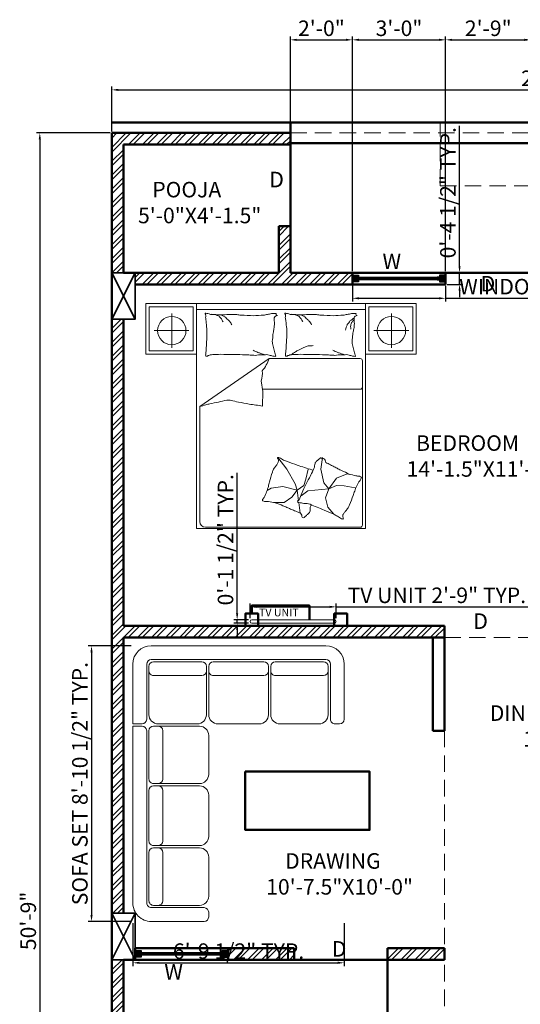
# Model space of a CAD drawing. Units: millimetres. Extents: x 67033 to 68301, y 155969 to 157209.
# Tile 4 of 17: x 67033 to 67226, y 156800 to 157181. Entities that reach past the tile are written whole.
import ezdxf

# ---------------------------------------------------------------- set-up
doc = ezdxf.new("R2010")
doc.units = ezdxf.units.MM
doc.linetypes.add('HIDDEN', pattern=[9.525, 6.35, -3.175])
for name, color, linetype, lineweight in [('A-ANNO-DIMS', 2, 'Continuous', 18), ('A-ANNO-TEXT', 7, 'Continuous', 18), ('A-AREA-IDEN', 3, 'Continuous', 18), ('A-COLS', 3, 'Continuous', 35), ('A-FLOR-OVHD', 1, 'HIDDEN', 18), ('A-FURN', 8, 'Continuous', 18), ('A-GLAZ', 4, 'Continuous', 25), ('A-WALL', 7, 'Continuous', 50), ('A-WALL-PATT', 8, 'Continuous', 13)]:
    doc.layers.add(name, color=color, linetype=linetype, lineweight=lineweight)
doc.styles.add('DIM_FONT', font='SIMPLEX.shx', dxfattribs={"width": 0.8})
doc.styles.get("Standard").update_dxf_attribs({"font": 'arial.ttf'})
doc.dimstyles.new('ISO-25', dxfattribs={"dimtxt": 6, "dimasz": 2.5, "dimexe": 1.25, "dimexo": 0.625, "dimtad": 1, "dimdec": 0, "dimlunit": 3, "dimtxsty": 'Standard', "dimcen": 2.5, "dimadec": 0, "dimazin": 0, "dimtfac": 1, "dimtdec": 0, "dimtmove": 0, "dimatfit": 3, "dimfxl": 1, "dimarcsym": 0})

# ---------------------------------------------------------------- blocks, each defined once
blk = doc.blocks.new('A$C79766A75')
for p, q in [((0.45, 1.9999), (0, 1.9999)), ((0, 1.9999), (0, 1.5499)), ((0.42, 1.9699), (0.03, 1.9699)), ((0.03, 1.9699), (0.03, 1.5799)), ((0.42, 1.5799), (0.42, 1.9699)), ((0.45, 1.5499), (0.45, 1.9999)), ((1.9506, 2), (0.4506, 2)), ((0.4506, 2), (0.4506, 0)), ((1.9506, 1.9476), (0.4506, 1.9476)), ((1.9506, 0), (1.9506, 2)), ((2.402, 1.9999), (1.952, 1.9999)), ((1.952, 1.9999), (1.952, 1.5499)), ((2.372, 1.9699), (1.982, 1.9699)), ((1.982, 1.9699), (1.982, 1.5799)), ((2.372, 1.5799), (2.372, 1.9699)), ((2.402, 1.5499), (2.402, 1.9999)), ((0.2304, 1.9125), (0.2304, 1.6061)), ((2.1824, 1.9125), (2.1824, 1.6061)), ((0.0743, 1.7595), (0.3834, 1.7595)), ((2.0263, 1.7595), (2.3354, 1.7595)), ((0.03, 1.5799), (0.42, 1.5799)), ((0.4234, 1.6034), (0.4228, 1.6034)), ((1.1461, 1.5617), (1.1254, 1.6443)), ((1.8553, 1.5617), (1.8346, 1.6443)), ((1.982, 1.5799), (2.372, 1.5799)), ((0, 1.5499), (0.45, 1.5499)), ((1.0972, 1.5115), (0.4791, 1.0841)), ((1.0972, 1.5115), (1.9048, 1.5115)), ((1.1536, 1.5317), (1.1461, 1.5617)), ((1.8628, 1.5317), (1.8553, 1.5617)), ((1.9248, 1.4915), (1.9248, 0.0322)), ((1.952, 1.5499), (2.402, 1.5499)), ((1.0383, 1.2184), (1.0246, 1.3138)), ((1.9048, 1.2389), (1.0354, 1.2389)), ((1.0365, 1.0883), (1.0383, 1.2184)), ((0.4791, 0.0622), (0.4791, 1.0841)), ((1.1731, 0.6316), (1.2523, 0.5276)), ((1.5696, 0.6317), (1.5559, 0.5286)), ((1.2523, 0.5276), (1.3274, 0.3973)), ((1.4223, 0.4407), (1.442, 0.5296)), ((1.5559, 0.5286), (1.5817, 0.4065)), ((1.4025, 0.3834), (1.4223, 0.4407)), ((1.6264, 0.355), (1.6952, 0.4478)), ((1.6952, 0.4478), (1.7898, 0.4856)), ((1.7898, 0.4856), (1.8139, 0.4822)), ((1.1139, 0.3597), (1.0779, 0.3397)), ((1.2167, 0.3736), (1.1139, 0.3597)), ((1.3452, 0.342), (1.2167, 0.3736)), ((1.3274, 0.3973), (1.3452, 0.342)), ((1.3452, 0.342), (1.4025, 0.3834)), ((1.4034, 0.3558), (1.3803, 0.2995)), ((1.6264, 0.355), (1.4406, 0.3361)), ((1.5817, 0.4065), (1.6264, 0.355)), ((1.5954, 0.2725), (1.6264, 0.355)), ((1.6264, 0.355), (1.6935, 0.3825)), ((1.6935, 0.3825), (1.7623, 0.379)), ((1.7623, 0.379), (1.8603, 0.3619)), ((1.8603, 0.3619), (1.8636, 0.3554)), ((1.2305, 0.2313), (1.2957, 0.2787)), ((1.2957, 0.2787), (1.3452, 0.342)), ((1.3452, 0.342), (1.3569, 0.2478)), ((1.3803, 0.2995), (1.3626, 0.256)), ((1.3907, 0.3), (1.3787, 0.2914)), ((1.4406, 0.3361), (1.3907, 0.3)), ((1.6161, 0.19), (1.5954, 0.2725)), ((1.1376, 0.2313), (1.2305, 0.2313)), ((1.3588, 0.2331), (1.3706, 0.1385)), ((1.6697, 0.1274), (1.6161, 0.19)), ((1.9048, 0.0122), (0.5291, 0.0122)), ((0.4506, 0), (1.9506, 0))]:
    blk.add_line(p, q)
for centre in [(0.2304, 1.7595), (2.1824, 1.7595)]:
    blk.add_circle(centre, 0.126)
for centre, radius, start, end in [((0.5232, 1.9139), 0.00342, 291.7883, 340.43603), ((0.525, 1.9085), 0.00232, 340.43603, 101.89306), ((0.5246, 1.9378), 0.0251, 274.30254, 291.7883), ((0.5311, 1.9093), 0.00428, 201.9904, 281.89306), ((0.4996, 1.8889), 0.0328, 338.57902, 8.13348), ((0.2896, 1.8253), 0.246, 8.13348, 12.10946), ((0.5465, 1.8994), 0.0156, 158.57902, 201.9904), ((0.7297, 1.8867), 0.1983, 187.6809, 192.10946), ((0.5486, 1.9393), 0.0289, 239.34875, 274.30254), ((1.4472, 1.8987), 0.9131, 183.36875, 187.6809), ((0.5458, 1.8568), 0.0539, 59.34875, 84.74081), ((0.546, 1.0829), 0.8208, 84.74081, 88.09211), ((0.6118, 2.0005), 0.0992, 254.06476, 274.21588), ((0.6775, 1.9817), 0.0992, 233.91364, 254.06476), ((0.6362, 0.406), 1.4943, 88.09211, 90.57574), ((0.7304, 1.9449), 0.0992, 216.17665, 233.91364), ((0.7737, 2.1075), 0.234, 242.76041, 249.13972), ((0.7661, 1.8961), 0.0992, 198.43965, 216.17665), ((0.7591, 1.0293), 0.8732, 90.57574, 94.80185), ((0.738, 1.949), 0.0768, 231.61143, 242.76041), ((0.974, 2.1633), 0.3916, 226.18849, 231.61143), ((0.9057, 1.9982), 0.2252, 219.03494, 226.18849), ((0.7631, 2.1919), 0.2897, 267.46141, 274.80185), ((0.8143, 2.0532), 0.1524, 259.81012, 267.46141), ((0.7515, 1.3747), 0.5293, 79.81012, 83.9133), ((0.8451, 0.8466), 1.049, 83.9133, 90), ((1.046, 1.2129), 0.6827, 90, 97.54685), ((1.1117, 1.6625), 0.2422, 97.54685, 105.74398), ((1.0352, 2.2041), 0.3048, 278.43719, 285.74398), ((1.1179, 2.0719), 0.1611, 270, 278.43719), ((1.171, 1.8579), 0.0342, 94.40021, 153.41948), ((1.6324, 1.8735), 0.4918, 180, 186.23236), ((1.1592, 2.0011), 0.0904, 258.72762, 270), ((1.1709, 1.9049), 0.0131, 153.41948, 258.72762), ((1.2325, 1.9139), 0.00342, 291.7883, 340.43603), ((1.2342, 1.9085), 0.00232, 340.43603, 101.89306), ((1.2338, 1.9378), 0.0251, 274.30254, 291.7883), ((1.2404, 1.9093), 0.00428, 201.9904, 281.89306), ((1.2088, 1.8889), 0.0328, 338.57902, 8.13348), ((0.9988, 1.8253), 0.246, 8.13348, 12.10946), ((1.2558, 1.8994), 0.0156, 158.57902, 201.9904), ((1.4389, 1.8867), 0.1983, 187.6809, 192.10946), ((1.2578, 1.9393), 0.0289, 239.34875, 274.30254), ((2.1565, 1.8987), 0.9131, 183.36875, 187.6809), ((1.2551, 1.8568), 0.0539, 59.34875, 84.74081), ((1.2552, 1.0829), 0.8208, 84.74081, 88.09211), ((1.3211, 2.0005), 0.0992, 254.06476, 274.21588), ((1.3868, 1.9817), 0.0992, 233.91364, 254.06476), ((1.3455, 0.406), 1.4943, 88.09211, 90.57574), ((1.4396, 1.9449), 0.0992, 216.17665, 233.91364), ((1.4829, 2.1075), 0.234, 242.76041, 249.13972), ((1.4753, 1.8961), 0.0992, 198.43965, 216.17665), ((1.4683, 1.0293), 0.8732, 90.57574, 94.80185), ((1.4473, 1.949), 0.0768, 231.61143, 242.76041), ((1.6833, 2.1633), 0.3916, 226.18849, 231.61143), ((1.615, 1.9982), 0.2252, 219.03494, 226.18849), ((1.4724, 2.1919), 0.2897, 267.46141, 274.80185), ((1.5236, 2.0532), 0.1524, 259.81012, 267.46141), ((1.4607, 1.3747), 0.5293, 79.81012, 83.9133), ((1.5543, 0.8466), 1.049, 83.9133, 90), ((1.7552, 1.2129), 0.6827, 90, 97.54685), ((1.821, 1.6625), 0.2422, 97.54685, 105.74398), ((1.7444, 2.2041), 0.3048, 278.43719, 285.74398), ((1.6908, 1.9123), 0.1399, 314.90238, 332.60117), ((1.7511, 1.9723), 0.1399, 297.20359, 314.90238), ((1.8271, 2.0719), 0.1611, 270, 278.43719), ((1.7896, 1.8667), 0.0526, 318.55709, 334.64488), ((1.784, 1.9167), 0.0899, 306.26407, 318.55709), ((1.8802, 1.8579), 0.0342, 94.40021, 153.41948), ((2.3416, 1.8735), 0.4918, 180, 186.23236), ((1.8684, 2.0011), 0.0904, 258.72762, 270), ((1.8802, 1.9049), 0.0131, 153.41948, 258.72762), ((1.2208, 1.7573), 0.6787, 178.36691, 183.36875), ((0.7932, 1.8591), 0.0493, 208.31676, 219.03494), ((0.9392, 1.9062), 0.2002, 203.00277, 208.31676), ((2.0027, 1.5994), 0.882, 167.80162, 170.31563), ((1.3446, 1.7858), 0.204, 170.31563, 180), ((1.9301, 1.7573), 0.6787, 178.36691, 183.36875), ((1.5025, 1.8591), 0.0493, 208.31676, 219.03494), ((1.6484, 1.9062), 0.2002, 203.00277, 208.31676), ((1.6404, 1.8023), 0.1399, 343.48502, 354.36887), ((1.6554, 1.8529), 0.1399, 332.60117, 343.48502), ((1.7653, 1.8132), 0.0562, 341.2201, 0), ((1.73, 1.7719), 0.0915, 0, 14.68511), ((1.6307, 1.8895), 0.2056, 338.18508, 341.2201), ((1.6887, 1.8881), 0.1511, 334.64488, 338.18508), ((2.7119, 1.5994), 0.882, 167.80162, 170.31563), ((2.0538, 1.7858), 0.204, 170.31563, 180), ((14.1519, 0.85), 13.6356, 176.49514, 176.94504), ((1.9066, 1.6447), 1.3652, 176.94504, 178.36691), ((0.4711, 1.7556), 0.6588, 351.99495, 357.33512), ((1.0578, 1.6474), 0.0677, 357.33512, 14.04519), ((0.8192, 1.792), 0.3171, 347.80162, 351.99495), ((14.8612, 0.85), 13.6356, 176.49514, 176.94504), ((2.6158, 1.6447), 1.3652, 176.94504, 178.36691), ((1.1803, 1.7556), 0.6588, 351.99495, 357.33512), ((1.767, 1.6474), 0.0677, 357.33512, 14.04519), ((1.5284, 1.792), 0.3171, 347.80162, 351.99495), ((0.8521, 1.5209), 0.3212, 170.00164, 176.49514), ((0.6583, 0.9067), 0.7387, 64.68893, 66.51559), ((1.5613, 1.5209), 0.3212, 170.00164, 176.49514), ((1.1895, 1.8508), 0.3126, 296.49848, 302.13498), ((0.7658, 2.8912), 1.4323, 294.32653, 296.49848), ((1.226, 2.0834), 0.5066, 290.67428, 294.32653), ((1.4305, 1.6796), 0.058, 274.08277, 290.67428), ((1.4679, 1.8969), 0.2721, 266.4448, 274.08277), ((1.3675, 0.9067), 0.7387, 64.68893, 66.51559), ((0.513, 1.535), 0.0193, 350.00164, 16.69777), ((0.5322, 1.5304), 0.00132, 16.69777, 97.12039), ((0.5579, 1.4467), 0.0875, 97.12039, 106.22115), ((0.5822, 1.4654), 0.0767, 106.22115, 117.28412), ((0.5507, 1.5832), 0.0453, 282.86904, 297.28412), ((0.5623, 1.6885), 0.1459, 273.57397, 282.86904), ((0.589, 2.7103), 1.164, 270.28654, 273.57397), ((0.7584, 7.2662), 5.7185, 269.02962, 270.28654), ((0.9401, 4.9065), 3.3622, 267.39037, 269.02962), ((0.9811, 2.7573), 1.2165, 265.38242, 267.39037), ((0.8583, 0.139), 1.4048, 85.38242, 87.25094), ((1.0175, 1.3138), 0.2301, 87.25094, 101.55856), ((0.7015, 0.888), 0.7387, 66.51559, 68.34226), ((0.7501, 0.8688), 0.7387, 68.34226, 70.57202), ((0.8043, 0.8497), 0.7387, 70.57202, 72.80178), ((1.0449, 1.6886), 0.1459, 263.56595, 281.55856), ((0.745, 1.6407), 0.3751, 320.35546, 339.85116), ((1.1099, 1.6599), 0.1197, 252.61359, 263.56595), ((1.0587, 1.3144), 0.2297, 72.61359, 80.5159), ((1.108, 1.2635), 0.2708, 80.5159, 85.91706), ((1.1535, 1.5308), 0.000917, 85.91706, 194.04494), ((1.2222, 1.535), 0.0193, 350.00164, 16.69777), ((1.2414, 1.5304), 0.00132, 16.69777, 97.12039), ((1.2671, 1.4467), 0.0875, 97.12039, 106.22115), ((1.2914, 1.4654), 0.0767, 106.22115, 117.28412), ((1.2599, 1.5832), 0.0453, 282.86904, 297.28412), ((1.2716, 1.6885), 0.1459, 273.57397, 282.86904), ((0.9025, 2.1618), 0.7286, 302.13498, 305.82629), ((1.2982, 2.7103), 1.164, 270.28654, 273.57397), ((1.4677, 7.2662), 5.7185, 269.02962, 270.28654), ((1.6493, 4.9065), 3.3622, 267.39037, 269.02962), ((1.6903, 2.7573), 1.2165, 265.38242, 267.39037), ((1.5676, 0.139), 1.4048, 85.38242, 87.25094), ((1.7268, 1.3138), 0.2301, 87.25094, 101.55856), ((1.4107, 0.888), 0.7387, 66.51559, 68.34226), ((1.4594, 0.8688), 0.7387, 68.34226, 70.57202), ((1.5136, 0.8497), 0.7387, 70.57202, 72.80178), ((1.7541, 1.6886), 0.1459, 263.56595, 281.55856), ((1.8192, 1.6599), 0.1197, 252.61359, 263.56595), ((1.7679, 1.3144), 0.2297, 72.61359, 80.5159), ((1.8172, 1.2635), 0.2708, 80.5159, 85.91706), ((1.8627, 1.5308), 0.000917, 85.91706, 194.04494), ((1.9048, 1.4915), 0.02, 0, 90), ((0.8556, 1.3759), 0.1801, 339.85116, 8.13558), ((1.9048, 1.2589), 0.02, 270, 0), ((-0.1888, 5.1029), 4.0646, 280.72756, 282.92554), ((0.7282, 1.1989), 0.0581, 262.26962, 280.72756), ((0.7833, 1.3309), 0.1942, 256.8096, 262.26962), ((0.2481, -1.3253), 2.5158, 76.8096, 78.32586), ((-0.0248, 2.8487), 1.8351, 285.93519, 287.73639), ((0.3872, 1.7415), 0.6574, 282.92554, 285.93519), ((0.3953, -1.4284), 2.588, 78.32586, 80.50498), ((0.413, -2.64), 3.7801, 80.50498, 82.308), ((1.1752, 0.6267), 0.0063, 166.71916, 233.42082), ((1.1734, 0.6272), 0.00443, 93.94836, 166.71916), ((1.163, 0.6103), 0.0142, 10.40739, 53.42082), ((1.1755, 0.5964), 0.0352, 69.65479, 93.94836), ((1.1011, 0.5989), 0.0771, 2.72862, 10.40739), ((1.1669, 0.5731), 0.0601, 51.41461, 69.65479), ((1.2538, 0.682), 0.0792, 231.41461, 247.29308), ((1.383, 0.7705), 0.2176, 307.21509, 313.52244), ((1.1426, 1.1456), 0.6605, 306.2163, 307.21509), ((1.7751, 0.3162), 0.3825, 126.2163, 127.52874), ((1.5806, 0.5924), 0.0452, 127.52874, 134.1274), ((1.5093, 0.6825), 0.0697, 308.81361, 314.1274), ((1.5706, 0.6318), 0.0127, 176.75451, 308.81361), ((1.5621, 0.59), 0.0359, 356.75451, 62.70976), ((1.3115, 0.4414), 0.1965, 153.92651, 162.1604), ((1.2077, 0.4922), 0.081, 140.29953, 153.92651), ((0.9961, 0.6678), 0.194, 320.29953, 329.09437), ((0.8605, 0.749), 0.352, 329.09437, 333.18207), ((1.1396, 0.6079), 0.0393, 333.18207, 345.42909), ((1.1628, 0.6019), 0.0153, 345.42909, 2.72862), ((1.5463, 1.3811), 0.8371, 247.29308, 249.87133), ((3.0113, 5.3783), 5.0942, 249.87133, 250.91638), ((2.374, 3.5362), 3.145, 250.91638, 253.39153), ((2.4089, 0.1204), 1.0054, 154.94715, 157.58378), ((1.5435, 0.5526), 0.0458, 157.58378, 188.04918), ((1.4828, 0.5833), 0.0226, 324.10643, 8.04918), ((1.4519, 0.6426), 0.0774, 313.52244, 324.10643), ((0.2201, -2.1858), 3.0972, 62.70976, 63.58535), ((2.5711, 2.3551), 2.0162, 242.50014, 243.58535), ((4.5245, 5.9445), 6.1019, 242.15178, 242.50014), ((-0.9881, -4.647), 5.8383, 62.15178, 62.50792), ((3.0311, -0.112), 2.003, 162.1604, 164.73746), ((2.8096, -0.3311), 1.5652, 150.06403, 152.91165), ((2.9813, -0.2643), 1.6868, 152.91165, 154.94715), ((1.5084, 0.6341), 0.1166, 253.39153, 259.26338), ((1.5182, -0.068), 0.6236, 62.50792, 69.25137), ((1.7121, 0.0657), 0.43, 69.25137, 77.37478), ((1.8682, 0.4049), 0.063, 77.37478, 93.38812), ((1.8955, 0.5247), 0.0599, 256.95977, 273.38812), ((1.8435, 0.4743), 0.0755, 310.50865, 333.66682), ((1.9257, 0.5082), 0.0509, 238.30826, 256.95977), ((1.9279, 0.441), 0.0168, 130.50865, 180.96136), ((1.9201, 0.4587), 0.0058, 180.96136, 238.30826), ((0.9098, 0.4035), 0.1798, 339.22273, 343.68776), ((0.5589, 0.5062), 0.5454, 343.68776, 346.159), ((2.6887, -0.0186), 1.6481, 164.73746, 166.159), ((1.2176, 0.4627), 0.2143, 330.06403, 337.76452), ((1.3456, 0.5261), 0.5454, 339.29188, 341.76311), ((1.701, 0.4319), 0.1798, 334.82685, 339.29188), ((-0.5166, 1.5491), 2.6619, 333.66682, 334.82685), ((1.0533, 0.2524), 0.0168, 134.90453, 185.35724), ((0.9882, 0.3177), 0.0755, 314.90453, 338.0627), ((-1.4109, 1.284), 2.6619, 338.0627, 339.22273), ((3.6966, -0.4634), 2.003, 157.76452, 160.34158), ((3.4079, -0.2212), 1.6481, 160.34158, 161.76311), ((1.0424, 0.2513), 0.0058, 185.35724, 242.70414), ((1.0631, 0.2914), 0.0509, 242.70414, 261.35565), ((1.0645, 0.3003), 0.0599, 261.35565, 277.784), ((1.0811, 0.1786), 0.063, 81.77066, 97.784), ((1.0286, -0.1846), 0.43, 73.64725, 81.77066), ((0.974, -0.3705), 0.6236, 66.9038, 73.64725), ((-1.0716, -5.1672), 5.8383, 66.54766, 66.9038), ((3.6805, 5.7866), 6.1019, 246.54766, 246.89602), ((1.3465, 0.2383), 0.00467, 287.18674, 70.62007), ((1.3486, 0.2247), 0.0092, 70.62007, 94.25932), ((1.3694, 0.234), 0.0231, 107.18674, 157.76452), ((1.3563, 0.267), 0.034, 262.01776, 274.25932), ((1.4091, 0.4221), 0.1955, 255.1193, 262.01776), ((1.358, 0.0507), 0.1794, 75.1193, 82.32164), ((1.4096, 0.153), 0.0712, 82.32164, 94.51184), ((1.4285, 0.2893), 0.0663, 261.87843, 274.51184), ((1.4755, 0.332), 0.1166, 248.99565, 261.87843), ((2.7121, 3.1012), 3.145, 246.5205, 248.99565), ((1.505, 0.1766), 0.0458, 161.97966, 192.44506), ((2.4175, -0.1202), 1.0054, 160.65521, 161.97966), ((1.856, 0.1288), 0.081, 135.90365, 149.53063), ((1.9797, 0.1108), 0.1965, 149.53063, 157.76452), ((2.0773, 2.0287), 2.0162, 246.89602, 247.98123), ((0.1602, -2.7118), 3.0972, 67.10564, 67.98123), ((1.3512, 0.1084), 0.0359, 1.15039, 67.10564), ((1.3997, 0.1094), 0.0127, 181.15039, 313.2095), ((1.3607, 0.1509), 0.0697, 313.2095, 318.52329), ((1.4468, 0.0748), 0.0452, 131.92462, 138.52329), ((1.6722, -0.1762), 0.3825, 130.61218, 131.92462), ((0.9933, 0.6156), 0.6605, 310.61218, 311.61098), ((1.2874, 0.2845), 0.2176, 311.61098, 317.91833), ((1.3914, 0.1905), 0.0774, 317.91833, 328.50231), ((1.4382, 0.1619), 0.0226, 328.50231, 12.44506), ((3.6993, 4.7998), 5.0942, 245.47545, 246.5205), ((2.051, 0.8725), 0.8371, 242.8972, 245.47545), ((1.7576, 0.1689), 0.0792, 227.01873, 242.8972), ((1.6963, 0.0438), 0.0601, 47.01873, 65.25891), ((1.737, 0.0526), 0.0352, 65.25891, 89.55248), ((1.7345, 0.1188), 0.0153, 341.03321, 358.33274), ((1.6723, 0.1058), 0.0771, 358.33274, 6.01151), ((1.7401, 0.0928), 0.0142, 6.01151, 49.02494), ((1.7162, 0.1388), 0.0393, 328.78619, 341.03321), ((1.756, 0.0832), 0.00443, 89.55248, 162.32327), ((1.4661, 0.3294), 0.352, 324.69849, 328.78619), ((1.7602, 0.0924), 0.0063, 162.32327, 229.02494), ((1.6279, 0.2819), 0.194, 315.90365, 324.69849), ((0.5291, 0.0622), 0.05, 180, 270), ((1.9048, 0.0322), 0.02, 270, 0)]:
    blk.add_arc(centre, radius, start, end)
at = {"style": 'DIM_FONT', "text_generation_flag": 4, "width": 0.8, "flags": 9}
for tag in ['XSIZE', 'YSIZE']:
    blk.add_attdef(tag, (1.9506, 2), '', height=0.0005, rotation=180, dxfattribs=at)
blk = doc.blocks.new('A$C2AFA021D')
for p, q in [((0.8, 2.3), (0.2, 2.3)), ((0.2, 2.15), (0.8, 2.15)), ((0.85, 2.2), (0.85, 2.25)), ((0, 2.1), (0, 0.2)), ((0.15, 0.2), (0.15, 2.1)), ((0.175, 1.55), (0.175, 2.075)), ((0.225, 2.125), (0.275, 2.125)), ((0.75, 2.125), (0.275, 2.125)), ((0.325, 2.075), (0.325, 1.55)), ((0.85, 1.6), (0.85, 2.025)), ((0.175, 0.875), (0.175, 1.425)), ((0.275, 1.5), (0.225, 1.5)), ((0.225, 1.475), (0.275, 1.475)), ((0.275, 1.5), (0.75, 1.5)), ((0.75, 1.475), (0.275, 1.475)), ((0.325, 1.425), (0.325, 0.875)), ((0.85, 0.925), (0.85, 1.375)), ((0.275, 0.825), (0.225, 0.825)), ((0.225, 0.8), (0.275, 0.8)), ((0.275, 0.825), (0.75, 0.825)), ((0.75, 0.8), (0.275, 0.8)), ((0.975, 0.825), (1.4, 0.825)), ((1.625, 0.825), (2.075, 0.825)), ((2.3, 0.825), (2.725, 0.825)), ((2.85, 0.2), (2.85, 0.775)), ((2.9, 0.825), (2.95, 0.825)), ((3, 0.775), (3, 0.2)), ((0.175, 0.225), (0.175, 0.75)), ((0.325, 0.75), (0.325, 0.225)), ((0.85, 0.275), (0.85, 0.7)), ((0.875, 0.275), (0.875, 0.725)), ((1.5, 0.725), (1.5, 0.275)), ((1.525, 0.275), (1.525, 0.725)), ((2.175, 0.725), (2.175, 0.275)), ((2.2, 0.275), (2.2, 0.725)), ((2.825, 0.725), (2.825, 0.275)), ((1.45, 0.325), (0.925, 0.325)), ((2.125, 0.325), (1.575, 0.325)), ((2.775, 0.325), (2.25, 0.325)), ((0.875, 0.275), (0.875, 0.225)), ((1.5, 0.225), (1.5, 0.275)), ((1.525, 0.275), (1.525, 0.225)), ((2.175, 0.225), (2.175, 0.275)), ((2.2, 0.275), (2.2, 0.225)), ((2.825, 0.225), (2.825, 0.275)), ((0.8, 0.15), (0.2, 0.15)), ((0.275, 0.175), (0.225, 0.175)), ((0.275, 0.175), (0.75, 0.175)), ((0.925, 0.175), (1.45, 0.175)), ((0.925, 0.15), (2.8, 0.15)), ((1.575, 0.175), (2.125, 0.175)), ((2.25, 0.175), (2.775, 0.175)), ((0.85, 0), (0.85, 0.1)), ((0.875, 0.1), (0.875, 0)), ((0.2, 0), (0.85, 0)), ((2.8, 0), (0.875, 0))]:
    blk.add_line(p, q)
for centre, radius, start, end in [((0.2, 2.1), 0.2, 90, 180), ((0.8, 2.25), 0.05, 0, 90), ((0.2, 2.1), 0.05, 90, 180), ((0.8, 2.2), 0.05, 270, 0), ((0.225, 2.075), 0.05, 90, 180), ((0.275, 2.075), 0.05, 0, 90), ((0.75, 2.025), 0.1, 0, 90), ((0.225, 1.55), 0.05, 180, 270), ((0.275, 1.55), 0.05, 270, 0), ((0.75, 1.6), 0.1, 270, 0), ((0.225, 1.425), 0.05, 90, 180), ((0.275, 1.425), 0.05, 0, 90), ((0.75, 1.375), 0.1, 360, 90), ((0.225, 0.875), 0.05, 180, 270), ((0.275, 0.875), 0.05, 270, 0), ((0.75, 0.925), 0.1, 270, 0), ((0.225, 0.75), 0.05, 90, 180), ((0.275, 0.75), 0.05, 0, 90), ((0.75, 0.7), 0.1, 0, 90), ((0.975, 0.725), 0.1, 90, 180), ((1.4, 0.725), 0.1, 0, 90), ((1.625, 0.725), 0.1, 90, 180), ((2.075, 0.725), 0.1, 0, 90), ((2.3, 0.725), 0.1, 90, 180), ((2.725, 0.725), 0.1, 0, 90), ((2.9, 0.775), 0.05, 90, 180), ((2.95, 0.775), 0.05, 0, 90), ((0.925, 0.275), 0.05, 90, 180), ((1.45, 0.275), 0.05, 360, 90), ((1.575, 0.275), 0.05, 90, 180), ((2.125, 0.275), 0.05, 360, 90), ((2.25, 0.275), 0.05, 90, 180), ((2.775, 0.275), 0.05, 360, 90), ((0.225, 0.225), 0.05, 180, 270), ((0.275, 0.225), 0.05, 270, 0), ((0.75, 0.275), 0.1, 270, 0), ((0.925, 0.225), 0.05, 180, 270), ((1.45, 0.225), 0.05, 270, 0), ((1.575, 0.225), 0.05, 180, 270), ((2.125, 0.225), 0.05, 270, 0), ((2.25, 0.225), 0.05, 180, 270), ((2.775, 0.225), 0.05, 270, 0), ((0.2, 0.2), 0.2, 180, 270), ((0.2, 0.2), 0.05, 180, 270), ((0.8, 0.1), 0.05, 0, 90), ((0.925, 0.1), 0.05, 90, 180), ((2.8, 0.2), 0.2, 270, 0), ((2.8, 0.2), 0.05, 270, 0)]:
    blk.add_arc(centre, radius, start, end)
blk = doc.blocks.new('*D30')
at = {"layer": 'A-ANNO-DIMS', "color": 0, "lineweight": -2, "transparency": 16777216}
for p, q in [((67068.44, 157137.62), (67068.44, 157154.9)), ((67407.44, 157137.82), (67407.44, 157154.9)), ((67070.94, 157153.65), (67404.94, 157153.65))]:
    blk.add_line(p, q, dxfattribs=at)
at = {"layer": 'A-ANNO-DIMS', "color": 0, "transparency": 16777216}
for points in [[(67070.94, 157154.06), (67070.94, 157153.23), (67068.44, 157153.65)], [(67404.94, 157154.06), (67404.94, 157153.23), (67407.44, 157153.65)]]:
    blk.add_solid(points, dxfattribs=at)
at = {"layer": 'Defpoints', "color": 0, "transparency": 16777216}
for p in [(67407.44, 157153.65), (67068.44, 157136.99), (67407.44, 157137.19)]:
    blk.add_point(p, dxfattribs=at)
at = {"layer": 'A-ANNO-DIMS', "color": 0, "transparency": 16777216, "insert": (67237.94, 157157.34), "char_height": 6, "attachment_point": 5}
blk.add_mtext('28\'-3"', dxfattribs=at)
blk = doc.blocks.new('*D31')
at = {"layer": 'A-ANNO-DIMS', "color": 0, "lineweight": -2, "transparency": 16777216}
for p, q in [((67067.81, 157136.99), (67039.34, 157136.99)), ((67040.59, 157134.49), (67040.59, 156530.49)), ((67067.81, 156527.99), (67039.34, 156527.99))]:
    blk.add_line(p, q, dxfattribs=at)
at = {"layer": 'A-ANNO-DIMS', "color": 0, "transparency": 16777216}
for points in [[(67040.17, 157134.49), (67041.01, 157134.49), (67040.59, 157136.99)], [(67040.17, 156530.49), (67041.01, 156530.49), (67040.59, 156527.99)]]:
    blk.add_solid(points, dxfattribs=at)
at = {"layer": 'Defpoints', "color": 0, "transparency": 16777216}
for p in [(67068.44, 157136.99), (67040.59, 156527.99), (67068.44, 156527.99)]:
    blk.add_point(p, dxfattribs=at)
at = {"layer": 'A-ANNO-DIMS', "color": 0, "transparency": 16777216, "insert": (67036.9, 156832.49), "char_height": 6, "attachment_point": 5, "rotation": 90}
blk.add_mtext('50\'-9"', dxfattribs=at)
blk = doc.blocks.new('WIN-900')
for p, q in [((3.67, 3.22), (33.2, 3.22)), ((3.67, 2.74), (33.2, 2.74)), ((33.2, 2.27), (3.67, 2.27))]:
    blk.add_line(p, q)
blk.add_lwpolyline([(0.44, 4.99), (36.44, 4.99), (36.44, 0.49), (0.44, 0.49)], close=True)
for points in [[(0.44, 4.09), (2.73, 4.09), (2.73, 3.22), (3.67, 3.22), (3.67, 2.27), (2.73, 2.27), (2.73, 1.4), (0.44, 1.4)], [(36.44, 4.09), (34.14, 4.09), (34.14, 3.22), (33.2, 3.22), (33.2, 2.27), (34.14, 2.27), (34.14, 1.4), (36.44, 1.4)]]:
    blk.add_lwpolyline(points)
blk = doc.blocks.new('COLUMN-230x460')
for p, q in [((0.44, 17.99), (9.44, -0.01)), ((9.44, 17.99), (0.44, -0.01))]:
    blk.add_line(p, q)
blk.add_lwpolyline([(0.44, 17.99), (9.44, 17.99), (9.44, -0.01), (0.44, -0.01)], close=True)
blk = doc.blocks.new('TV-UNIT')
for points in [[(0.68, 1.36), (32.57, 1.36)], [(32.57, 0), (0.68, 0)]]:
    blk.add_lwpolyline(points)
for centre, start, end in [((0.68, 0.68), 90, 270), ((32.57, 0.68), 270, 90)]:
    blk.add_arc(centre, 0.678, start, end)
blk = doc.blocks.new('*D51')
at = {"layer": 'A-ANNO-DIMS', "color": 0, "lineweight": -2, "transparency": 16777216}
for p, q in [((67161.44, 157077.87), (67161.44, 157071.84)), ((67197.44, 157077.87), (67197.44, 157071.84)), ((67163.94, 157073.09), (67194.94, 157073.09)), ((67197.44, 157073.09), (67287.35, 157073.09))]:
    blk.add_line(p, q, dxfattribs=at)
at = {"layer": 'A-ANNO-DIMS', "color": 0, "transparency": 16777216}
for points in [[(67163.94, 157073.51), (67163.94, 157072.68), (67161.44, 157073.09)], [(67194.94, 157073.51), (67194.94, 157072.68), (67197.44, 157073.09)]]:
    blk.add_solid(points, dxfattribs=at)
at = {"layer": 'Defpoints', "color": 0, "transparency": 16777216}
for p in [(67161.44, 157078.49), (67197.44, 157078.49), (67197.44, 157073.09)]:
    blk.add_point(p, dxfattribs=at)
at = {"layer": 'A-ANNO-DIMS', "color": 0, "transparency": 16777216, "insert": (67243.64, 157076.83), "char_height": 6, "attachment_point": 5}
blk.add_mtext('WINDOW W 3\'-0" TYP.', dxfattribs=at)
blk = doc.blocks.new('*D52')
at = {"layer": 'A-ANNO-DIMS', "color": 0, "lineweight": -2, "transparency": 16777216}
for p, q in [((67202.84, 157085.49), (67202.84, 157139.8)), ((67198.06, 157082.99), (67204.09, 157082.99)), ((67202.84, 157078.49), (67202.84, 157082.99)), ((67198.06, 157078.49), (67204.09, 157078.49)), ((67202.84, 157075.99), (67202.84, 157073.49))]:
    blk.add_line(p, q, dxfattribs=at)
at = {"layer": 'A-ANNO-DIMS', "color": 0, "transparency": 16777216}
for points in [[(67202.42, 157085.49), (67203.25, 157085.49), (67202.84, 157082.99)], [(67202.42, 157075.99), (67203.25, 157075.99), (67202.84, 157078.49)]]:
    blk.add_solid(points, dxfattribs=at)
at = {"layer": 'Defpoints', "color": 0, "transparency": 16777216}
for p in [(67197.44, 157082.99), (67202.84, 157082.99), (67197.44, 157078.49)]:
    blk.add_point(p, dxfattribs=at)
at = {"layer": 'A-ANNO-DIMS', "color": 0, "transparency": 16777216, "insert": (67199.11, 157113.9), "char_height": 6, "attachment_point": 5, "rotation": 90}
blk.add_mtext('0\'-4 1/2" TYP.', dxfattribs=at)
blk = doc.blocks.new('*D65')
at = {"layer": 'A-ANNO-DIMS', "color": 0, "lineweight": -2, "transparency": 16777216}
for p, q in [((67075.94, 156938.81), (67059.34, 156938.81)), ((67060.59, 156936.31), (67060.59, 156834.77)), ((67075.94, 156832.27), (67059.34, 156832.27))]:
    blk.add_line(p, q, dxfattribs=at)
at = {"layer": 'A-ANNO-DIMS', "color": 0, "transparency": 16777216}
for points in [[(67060.17, 156936.31), (67061, 156936.31), (67060.59, 156938.81)], [(67060.17, 156834.77), (67061, 156834.77), (67060.59, 156832.27)]]:
    blk.add_solid(points, dxfattribs=at)
at = {"layer": 'Defpoints', "color": 0, "transparency": 16777216}
for p in [(67076.57, 156938.81), (67060.59, 156832.27), (67076.57, 156832.27)]:
    blk.add_point(p, dxfattribs=at)
at = {"layer": 'A-ANNO-DIMS', "color": 0, "transparency": 16777216, "insert": (67056.86, 156885.54), "char_height": 6, "attachment_point": 5, "rotation": 90}
blk.add_mtext('SOFA SET 8\'-10 1/2" TYP.', dxfattribs=at)
blk = doc.blocks.new('*D66')
at = {"layer": 'A-ANNO-DIMS', "color": 0, "lineweight": -2, "transparency": 16777216}
for p, q in [((67076.57, 156831.65), (67076.57, 156815.04)), ((67158.25, 156831.65), (67158.25, 156815.04)), ((67079.07, 156816.29), (67155.75, 156816.29))]:
    blk.add_line(p, q, dxfattribs=at)
at = {"layer": 'A-ANNO-DIMS', "color": 0, "transparency": 16777216}
for points in [[(67079.07, 156816.71), (67079.07, 156815.87), (67076.57, 156816.29)], [(67155.75, 156816.71), (67155.75, 156815.87), (67158.25, 156816.29)]]:
    blk.add_solid(points, dxfattribs=at)
at = {"layer": 'Defpoints', "color": 0, "transparency": 16777216}
for p in [(67076.57, 156832.27), (67158.25, 156832.27), (67158.25, 156816.29)]:
    blk.add_point(p, dxfattribs=at)
at = {"layer": 'A-ANNO-DIMS', "color": 0, "transparency": 16777216, "insert": (67117.41, 156820.02), "char_height": 6, "attachment_point": 5}
blk.add_mtext('6\'-9 1/2" TYP.', dxfattribs=at)
blk = doc.blocks.new('*D77')
at = {"layer": 'A-ANNO-DIMS', "color": 0, "lineweight": -2, "transparency": 16777216}
for p, q in [((67121.85, 156949.49), (67121.85, 156955.1)), ((67124.35, 156953.85), (67152.6, 156953.85)), ((67155.1, 156949.49), (67155.1, 156955.1)), ((67155.1, 156953.85), (67230.5, 156953.85))]:
    blk.add_line(p, q, dxfattribs=at)
at = {"layer": 'A-ANNO-DIMS', "color": 0, "transparency": 16777216}
for points in [[(67124.35, 156954.27), (67124.35, 156953.43), (67121.85, 156953.85)], [(67152.6, 156954.27), (67152.6, 156953.43), (67155.1, 156953.85)]]:
    blk.add_solid(points, dxfattribs=at)
at = {"layer": 'Defpoints', "color": 0, "transparency": 16777216}
for p in [(67155.1, 156953.85), (67121.85, 156948.86), (67155.1, 156948.86)]:
    blk.add_point(p, dxfattribs=at)
at = {"layer": 'A-ANNO-DIMS', "color": 0, "transparency": 16777216, "insert": (67194.05, 156957.54), "char_height": 6, "attachment_point": 5}
blk.add_mtext('TV UNIT 2\'-9" TYP.', dxfattribs=at)
blk = doc.blocks.new('*D78')
at = {"layer": 'A-ANNO-DIMS', "color": 0, "lineweight": -2, "transparency": 16777216}
for p, q in [((67116.87, 156951.36), (67116.87, 157005.67)), ((67121.23, 156948.86), (67115.62, 156948.86)), ((67121.23, 156947.51), (67115.62, 156947.51)), ((67116.87, 156947.51), (67116.87, 156948.86)), ((67116.87, 156945.01), (67116.87, 156942.51))]:
    blk.add_line(p, q, dxfattribs=at)
at = {"layer": 'A-ANNO-DIMS', "color": 0, "transparency": 16777216}
for points in [[(67116.45, 156951.36), (67117.28, 156951.36), (67116.87, 156948.86)], [(67116.45, 156945.01), (67117.28, 156945.01), (67116.87, 156947.51)]]:
    blk.add_solid(points, dxfattribs=at)
at = {"layer": 'Defpoints', "color": 0, "transparency": 16777216}
for p in [(67116.87, 156948.86), (67121.85, 156948.86), (67121.85, 156947.51)]:
    blk.add_point(p, dxfattribs=at)
at = {"layer": 'A-ANNO-DIMS', "color": 0, "transparency": 16777216, "insert": (67113.14, 156979.77), "char_height": 6, "attachment_point": 5, "rotation": 90}
blk.add_mtext('0\'-1 1/2" TYP.', dxfattribs=at)
blk = doc.blocks.new('*D79')
at = {"layer": 'A-ANNO-DIMS', "color": 0, "lineweight": -2, "transparency": 16777216}
for p, q in [((67137.44, 157083.62), (67137.44, 157174.24)), ((67161.44, 157083.62), (67161.44, 157174.24)), ((67139.94, 157172.99), (67158.94, 157172.99))]:
    blk.add_line(p, q, dxfattribs=at)
at = {"layer": 'A-ANNO-DIMS', "color": 0, "transparency": 16777216}
for points in [[(67139.94, 157173.41), (67139.94, 157172.58), (67137.44, 157172.99)], [(67158.94, 157173.41), (67158.94, 157172.58), (67161.44, 157172.99)]]:
    blk.add_solid(points, dxfattribs=at)
at = {"layer": 'Defpoints', "color": 0, "transparency": 16777216}
for p in [(67161.44, 157172.99), (67137.44, 157082.99), (67161.44, 157082.99)]:
    blk.add_point(p, dxfattribs=at)
at = {"layer": 'A-ANNO-DIMS', "color": 0, "transparency": 16777216, "insert": (67149.44, 157176.68), "char_height": 6, "attachment_point": 5}
blk.add_mtext('2\'-0"', dxfattribs=at)
blk = doc.blocks.new('*D80')
at = {"layer": 'A-ANNO-DIMS', "color": 0, "lineweight": -2, "transparency": 16777216}
for p, q in [((67161.44, 157083.62), (67161.44, 157174.24)), ((67197.44, 157083.62), (67197.44, 157174.24)), ((67163.94, 157172.99), (67194.94, 157172.99))]:
    blk.add_line(p, q, dxfattribs=at)
at = {"layer": 'A-ANNO-DIMS', "color": 0, "transparency": 16777216}
for points in [[(67163.94, 157173.41), (67163.94, 157172.58), (67161.44, 157172.99)], [(67194.94, 157173.41), (67194.94, 157172.58), (67197.44, 157172.99)]]:
    blk.add_solid(points, dxfattribs=at)
at = {"layer": 'Defpoints', "color": 0, "transparency": 16777216}
for p in [(67197.44, 157172.99), (67161.44, 157082.99), (67197.44, 157082.99)]:
    blk.add_point(p, dxfattribs=at)
at = {"layer": 'A-ANNO-DIMS', "color": 0, "transparency": 16777216, "insert": (67179.44, 157176.68), "char_height": 6, "attachment_point": 5}
blk.add_mtext('3\'-0"', dxfattribs=at)
blk = doc.blocks.new('*D81')
at = {"layer": 'A-ANNO-DIMS', "color": 0, "lineweight": -2, "transparency": 16777216}
for p, q in [((67197.44, 157083.62), (67197.44, 157174.24)), ((67230.44, 157083.62), (67230.44, 157174.24)), ((67199.94, 157172.99), (67227.94, 157172.99))]:
    blk.add_line(p, q, dxfattribs=at)
at = {"layer": 'A-ANNO-DIMS', "color": 0, "transparency": 16777216}
for points in [[(67199.94, 157173.41), (67199.94, 157172.58), (67197.44, 157172.99)], [(67227.94, 157173.41), (67227.94, 157172.58), (67230.44, 157172.99)]]:
    blk.add_solid(points, dxfattribs=at)
at = {"layer": 'Defpoints', "color": 0, "transparency": 16777216}
for p in [(67230.44, 157172.99), (67197.44, 157082.99), (67230.44, 157082.99)]:
    blk.add_point(p, dxfattribs=at)
at = {"layer": 'A-ANNO-DIMS', "color": 0, "transparency": 16777216, "insert": (67213.94, 157176.68), "char_height": 6, "attachment_point": 5}
blk.add_mtext('2\'-9"', dxfattribs=at)

msp = doc.modelspace()

# ---------------------------------------------------------------- hatches: boundary and pattern name
at = {"layer": 'A-GLAZ'}
h = msp.add_hatch(color=256, dxfattribs=at)
h.dxf.hatch_style = 1
h.paths.add_polyline_path([(67164.67, 157081.22), (67163.73, 157081.22), (67163.73, 157082.09), (67161.44, 157082.09), (67161.44, 157079.4), (67163.73, 157079.4), (67163.73, 157080.27), (67164.67, 157080.27)])
h = msp.add_hatch(color=256, dxfattribs=at)
h.dxf.hatch_style = 1
h.paths.add_polyline_path([(67197.44, 157082.09), (67195.14, 157082.09), (67195.14, 157081.22), (67194.2, 157081.22), (67194.2, 157080.27), (67195.14, 157080.27), (67195.14, 157079.4), (67197.44, 157079.4)], flags=17)
h = msp.add_hatch(color=256, dxfattribs=at)
h.dxf.hatch_style = 1
h.paths.add_polyline_path([(67080.67, 156820.22), (67079.73, 156820.22), (67079.73, 156821.09), (67077.44, 156821.09), (67077.44, 156818.4), (67079.73, 156818.4), (67079.73, 156819.27), (67080.67, 156819.27)])
h = msp.add_hatch(color=256, dxfattribs=at)
h.dxf.hatch_style = 1
h.paths.add_polyline_path([(67113.44, 156821.09), (67111.14, 156821.09), (67111.14, 156820.22), (67110.2, 156820.22), (67110.2, 156819.27), (67111.14, 156819.27), (67111.14, 156818.4), (67113.44, 156818.4)])
at = {"layer": 'A-WALL-PATT'}
h = msp.add_hatch(dxfattribs=at)
h.set_pattern_fill('ANSI32', color=256, scale=0.4)
h.paths.add_polyline_path([(67072.94, 157132.49), (67137.44, 157132.49), (67137.44, 157136.99), (67068.44, 157136.99), (67068.44, 157082.99), (67072.94, 157082.99)])
h = msp.add_hatch(dxfattribs=at)
h.set_pattern_fill('ANSI32', color=256, scale=0.4)
h.paths.add_polyline_path([(67161.44, 157082.99), (67137.44, 157082.99), (67137.44, 157100.99), (67132.94, 157100.99), (67132.94, 157082.99), (67077.44, 157082.99), (67077.44, 157078.49), (67161.44, 157078.49)])
h = msp.add_hatch(dxfattribs=at)
h.set_pattern_fill('ANSI32', color=256, scale=0.4)
h.paths.add_polyline_path([(67072.94, 157064.99), (67068.44, 157064.99), (67068.44, 156835.49), (67072.94, 156835.49), (67072.94, 156941.99), (67196.98, 156941.99), (67196.98, 156946.49), (67072.94, 156946.49)])
h = msp.add_hatch(dxfattribs=at)
h.set_pattern_fill('ANSI32', color=256, scale=0.4)
h.paths.add_polyline_path([(67138.94, 156821.99), (67113.44, 156821.99), (67113.44, 156817.49), (67138.94, 156817.49)])
h = msp.add_hatch(dxfattribs=at)
h.set_pattern_fill('ANSI32', color=256, scale=0.4)
h.paths.add_polyline_path([(67196.98, 156821.99), (67174.94, 156821.99), (67174.94, 156817.49), (67196.98, 156817.49)])
h = msp.add_hatch(dxfattribs=at)
h.set_pattern_fill('ANSI32', color=256, scale=0.4)
h.paths.add_polyline_path([(67072.94, 156817.49), (67068.44, 156817.49), (67068.44, 156640.48), (67072.94, 156640.48)])

# ---------------------------------------------------------------- linework, layer by layer
at = {"layer": 'A-FLOR-OVHD'}
for p, q in [((67195.36, 157116.61), (67195.36, 157140.99)), ((67137.44, 157136.99), (67405.1, 157136.99)), ((67195.36, 157116.61), (67402.94, 157116.61)), ((67196.98, 156941.99), (67230.44, 156941.99)), ((67196.98, 156905.99), (67196.98, 156821.99)), ((67196.98, 156770.99), (67196.98, 156817.49))]:
    msp.add_line(p, q, dxfattribs=at)
at = {"layer": 'A-WALL'}
for p, q in [((67068.44, 157140.99), (67407.44, 157140.99)), ((67137.44, 157140.99), (67137.44, 157082.99)), ((67068.44, 157136.99), (67068.44, 156527.99)), ((67137.44, 157136.99), (67068.44, 157136.99)), ((67072.94, 157132.49), (67072.94, 157082.99)), ((67072.94, 157132.49), (67137.44, 157132.49)), ((67137.44, 157132.99), (67402.94, 157132.99)), ((67132.94, 157100.99), (67132.94, 157082.99)), ((67132.94, 157100.99), (67137.44, 157100.99)), ((67072.94, 157082.99), (67132.94, 157082.99)), ((67137.44, 157082.99), (67197.44, 157082.99)), ((67161.44, 157082.99), (67161.44, 157078.49)), ((67197.44, 157082.99), (67197.44, 157078.49)), ((67197.44, 157082.99), (67230.44, 157082.99)), ((67077.44, 157078.49), (67197.44, 157078.49)), ((67072.94, 157064.99), (67072.94, 156946.49)), ((67072.94, 156946.49), (67196.98, 156946.49)), ((67196.98, 156946.49), (67196.98, 156905.99)), ((67072.94, 156941.99), (67196.98, 156941.99)), ((67072.94, 156941.99), (67072.94, 156835.49)), ((67192.48, 156941.99), (67192.48, 156905.99)), ((67192.48, 156905.99), (67196.98, 156905.99)), ((67077.44, 156821.99), (67138.94, 156821.99)), ((67077.44, 156821.99), (67077.44, 156817.49)), ((67113.44, 156821.99), (67113.44, 156817.49)), ((67138.94, 156821.99), (67138.94, 156817.49)), ((67174.94, 156821.99), (67174.94, 156622.49)), ((67174.94, 156821.99), (67196.98, 156821.99)), ((67196.98, 156821.99), (67196.98, 156817.49)), ((67072.94, 156817.49), (67138.94, 156817.49)), ((67072.94, 156817.49), (67072.94, 156640.48)), ((67174.94, 156817.49), (67138.94, 156817.49)), ((67174.94, 156817.49), (67196.98, 156817.49))]:
    msp.add_line(p, q, dxfattribs=at)
msp.add_lwpolyline([(67122.53, 156951.23), (67122.53, 156954.35), (67144.78, 156954.35), (67144.78, 156948.86)], dxfattribs=at)
for points in [[(67120.08, 156946.49), (67124.99, 156946.49), (67124.99, 156951.23), (67120.08, 156951.23)], [(67154.43, 156946.49), (67159.34, 156946.49), (67159.34, 156951.23), (67154.43, 156951.23)], [(67119.98, 156890.16), (67168.06, 156890.16), (67168.06, 156867.66), (67119.98, 156867.66)]]:
    msp.add_lwpolyline(points, close=True, dxfattribs=at)

# ---------------------------------------------------------------- block references
at = {"layer": 'A-COLS'}
for p in [(67068, 157065), (67068, 156817.5)]:
    msp.add_blockref('COLUMN-230x460', p, dxfattribs=at)
at = {"layer": 'A-FURN', "xscale": 43.50257579484658, "yscale": 43.50257579484658, "zscale": 43.50257579484658}
msp.add_blockref('A$C79766A75', (67081.58, 156984.08), dxfattribs=at)
at = {"layer": 'A-FURN'}
msp.add_blockref('TV-UNIT', (67121.85, 156947.51), dxfattribs=at)
at = {"layer": 'A-FURN', "xscale": 35.51344104378158, "yscale": 35.51344104378158, "zscale": 35.51344104378158, "rotation": 270}
msp.add_blockref('A$C2AFA021D', (67076.57, 156938.81), dxfattribs=at)
at = {"layer": 'A-GLAZ'}
for p in [(67161, 157078), (67077, 156817)]:
    msp.add_blockref('WIN-900', p, dxfattribs=at)

# ---------------------------------------------------------------- texts
at = {"layer": 'A-ANNO-TEXT', "attachment_point": 1}
for s, width, insert, char_height in [('   D', 19.5287, (67123.81, 157121.99), 6), ('   W', 19.5287, (67167.56, 157090.37), 6), ('   D', 19.5287, (67205.51, 157081.74), 6), ('  TV UNIT', 25.6344, (67123.5, 156953.18), 3), ('   D', 19.5287, (67202.67, 156951.32), 6), ('   D', 19.5287, (67147.98, 156824.67), 6), ('   W', 19.5287, (67083.23, 156815.8), 6)]:
    msp.add_mtext_dynamic_manual_height_columns(s, width=width, gutter_width=12.5, heights=[0], dxfattribs=dict(at, insert=insert, char_height=char_height))
at = {"layer": 'A-AREA-IDEN', "char_height": 6, "attachment_point": 1}
for s, width, insert in [('       POOJA \\P    5\'-0"X4\'-1.5"', 59.4046, (67071.23, 157118.1)), ('  BEDROOM \\P14\'-1.5"X11\'-0"', 59.4046, (67182.37, 157020.14)), ('  DINNING/ FAMILY LOUNGE\\P         13\'-3"X13\'-10.5"', 118.0294, (67210.86, 156915.79)), ('       DRAWING\\P   10\'-7.5"X10\'-0"', 75.351, (67122.59, 156858.65))]:
    msp.add_mtext_dynamic_manual_height_columns(s, width=width, gutter_width=12.5, heights=[0], dxfattribs=dict(at, insert=insert))

# ---------------------------------------------------------------- dimensions: what is measured, and where the dimension line sits
at = {"layer": 'A-ANNO-DIMS'}
for base, p1, p2, override, picture, middle in [((67161.44, 157172.99), (67137.44, 157082.99), (67161.44, 157082.99), {"dimdec": 1, "dimlfac": 1, "dimrnd": 0, "dimzin": 1, "dimdsep": 46, "dimlunit": 4, "dimfrac": 2}, '*D79', (67149.44, 157176.68)), ((67197.44, 157172.99), (67161.44, 157082.99), (67197.44, 157082.99), {"dimdec": 1, "dimlfac": 1, "dimrnd": 0, "dimzin": 1, "dimdsep": 46, "dimlunit": 4, "dimfrac": 2}, '*D80', (67179.44, 157176.68)), ((67230.44, 157172.99), (67197.44, 157082.99), (67230.44, 157082.99), {"dimdec": 1, "dimlfac": 1, "dimrnd": 0, "dimzin": 1, "dimdsep": 46, "dimlunit": 4, "dimfrac": 2}, '*D81', (67213.94, 157176.68)), ((67407.44, 157153.65), (67068.44, 157136.99), (67407.44, 157137.19), {"dimclrd": 0, "dimclre": 0, "dimclrt": 0}, '*D30', (67237.94, 157157.34))]:
    dim = msp.add_linear_dim(base=base, p1=p1, p2=p2, dimstyle='ISO-25', override=override, dxfattribs=at)
    dim.commit()
    dim.dimension.update_dxf_attribs({"geometry": picture, "text_midpoint": middle})
for base, p1, p2, angle, text, picture, middle in [((67202.84, 157082.99), (67197.44, 157078.49), (67197.44, 157082.99), 90, '<> TYP.', '*D52', (67199.11, 157113.9)), ((67116.8675, 156948.8642), (67121.8549, 156947.5078), (67121.8549, 156948.8642), 90, '<> TYP.', '*D78', (67113.1401, 156979.7661)), ((67060.59, 156832.27), (67076.57, 156938.81), (67076.57, 156832.27), 270, 'SOFA SET <> TYP.', '*D65', (67056.86, 156885.54))]:
    dim = msp.add_linear_dim(base=base, p1=p1, p2=p2, angle=angle, text=text, dimstyle='ISO-25', override={"dimdec": 1, "dimrnd": 0, "dimzin": 1, "dimlunit": 4, "dimfrac": 2}, dxfattribs=at)
    dim.commit()
    dim.dimension.update_dxf_attribs({"geometry": picture, "text_midpoint": middle})
dim = msp.add_linear_dim(base=(67040.59, 156527.99), p1=(67068.44, 157136.99), p2=(67068.44, 156527.99), angle=90, dimstyle='ISO-25', override={"dimclrd": 0, "dimclre": 0, "dimclrt": 0}, dxfattribs=at)
dim.commit()
dim.dimension.update_dxf_attribs({"geometry": '*D31', "text_midpoint": (67036.9, 156832.49)})
for base, p1, p2, text, picture, middle in [((67197.44, 157073.09), (67161.44, 157078.49), (67197.44, 157078.49), 'WINDOW W <> TYP.', '*D51', (67243.64, 157076.83)), ((67155.1043, 156953.8516), (67121.8549, 156948.8642), (67155.1043, 156948.8642), 'TV UNIT <> TYP.', '*D77', (67194.0534, 156957.54)), ((67158.25, 156816.29), (67076.57, 156832.27), (67158.25, 156832.27), '<> TYP.', '*D66', (67117.41, 156820.02))]:
    dim = msp.add_linear_dim(base=base, p1=p1, p2=p2, text=text, dimstyle='ISO-25', override={"dimdec": 1, "dimrnd": 0, "dimzin": 1, "dimlunit": 4, "dimfrac": 2}, dxfattribs=at)
    dim.commit()
    dim.dimension.update_dxf_attribs({"geometry": picture, "text_midpoint": middle})

doc.saveas('drawing.dxf')
